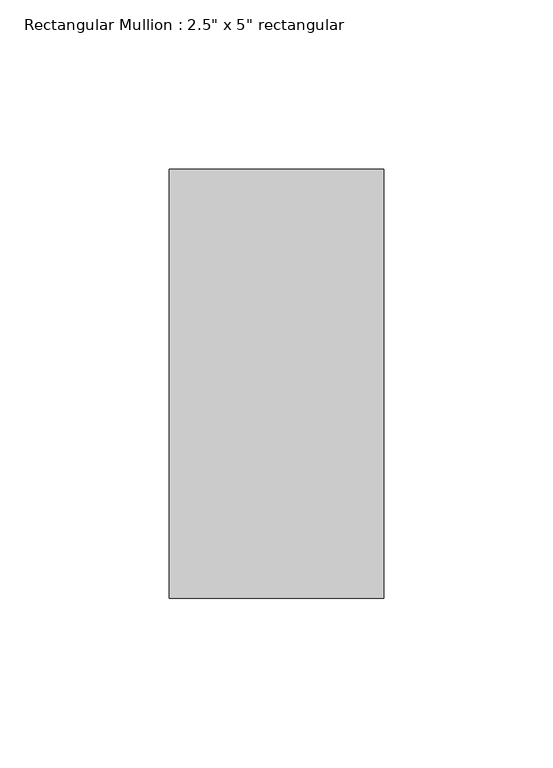
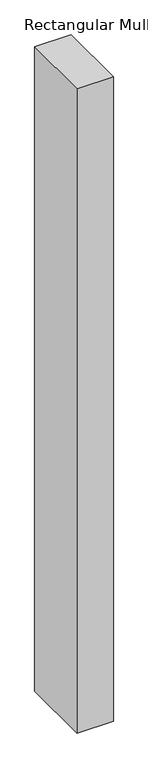
"""IFC4 building model written with IfcOpenShell, lengths in millimetres: member geometry."""

from ifc_helpers import new_model, si_unit, frame, origin, place, context, project, spatial, polyline, outline, extrude, source, transform, mapped, element, save


def member_fed28cdb(model_context):
    return source(origin(), model_context, "Body", "SweptSolid", [
        extrude(outline(polyline([(31.75, 63.5), (31.75, -63.5), (-31.75, -63.5), (-31.75, 63.5), (31.75, 63.5)])), frame((0.0, 0.0, -1185.3333333), z_axis=(0.0, 0.0, 1.0), x_axis=(1.0, 0.0, 0.0)), (0.0, 0.0, 1.0), 1185.3333333),
    ])


if __name__ == "__main__":
    model = new_model("IFC4")
    model_context = context("Model", 3, world=origin())
    ifc_project = project(units=[si_unit("LENGTHUNIT", "METRE", prefix="MILLI")], contexts=[model_context])
    site = spatial("IfcSite", under=ifc_project)
    building = spatial("IfcBuilding", under=site)
    placement = place(None, origin())
    member_shape = member_fed28cdb(model_context)
    element("IfcMember", 1, ObjectType="Rectangular Mullion : 2.5\" x 5\" rectangular", at=placement, inside=building, context=model_context, shape_type="MappedRepresentation", body=[
        mapped(member_shape, transform((0.0, 0.0, 0.0), x_axis=(1.0, 0.0, 0.0), y_axis=(0.0, 1.0, 0.0), z_axis=(0.0, 0.0, 1.0))),
    ])
    save(model, "model.ifc")

# Revit data of these elements
# Type "Rectangular Mullion : 2.5\" x 5\" rectangular"
#   built-in parameter 1007304 = 0.416667 (stored number, unit not read)
#   built-in parameter 1007301 = 0.104167 (stored number, unit not read)
#   built-in parameter 1007300 = 0.104167 (stored number, unit not read)
# Element 1 (IfcMember, "Rectangular Mullion : 2.5\" x 5\" rectangular")
#   Materials on its faces: "Aluminum"
# Materials
#   "Aluminum": class "Metal", colour RGB 247 247 247, transparency 0, Description = "Aluminum 6061", Cost = 0
